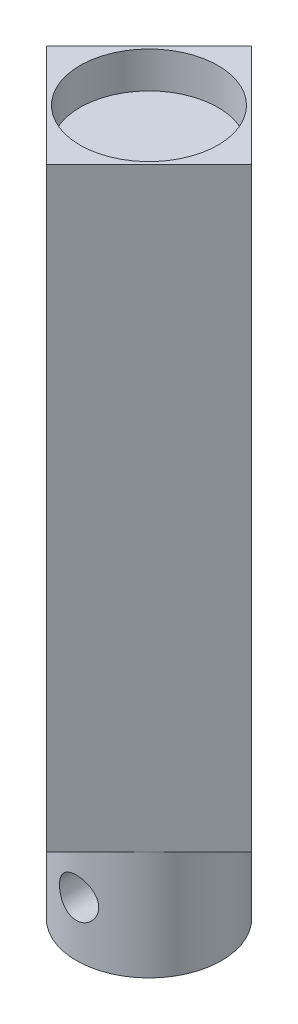
ISO-10303-21;
HEADER;
FILE_DESCRIPTION(('STEP AP214'),'2;1');
FILE_NAME('part.step','',(''),(''),'','','');
FILE_SCHEMA(('AUTOMOTIVE_DESIGN { 1 0 10303 214 1 1 1 1 }'));
ENDSEC;
DATA;
#1=APPLICATION_CONTEXT('core data for automotive mechanical design processes');
#2=APPLICATION_PROTOCOL_DEFINITION('international standard','automotive_design',2000,#1);
#3=PRODUCT_CONTEXT('',#1,'mechanical');
#4=PRODUCT('Part','Part','',(#3));
#5=PRODUCT_RELATED_PRODUCT_CATEGORY('part','',(#4));
#6=PRODUCT_DEFINITION_FORMATION('','',#4);
#7=PRODUCT_DEFINITION_CONTEXT('part definition',#1,'design');
#8=PRODUCT_DEFINITION('design','',#6,#7);
#9=PRODUCT_DEFINITION_SHAPE('','',#8);
#10=(LENGTH_UNIT() NAMED_UNIT(*) SI_UNIT(.MILLI.,.METRE.));
#11=(NAMED_UNIT(*) PLANE_ANGLE_UNIT() SI_UNIT($,.RADIAN.));
#12=(NAMED_UNIT(*) SI_UNIT($,.STERADIAN.) SOLID_ANGLE_UNIT());
#13=UNCERTAINTY_MEASURE_WITH_UNIT(LENGTH_MEASURE(1.E-05),#10,'distance_accuracy_value','');
#14=(GEOMETRIC_REPRESENTATION_CONTEXT(3) GLOBAL_UNCERTAINTY_ASSIGNED_CONTEXT((#13)) GLOBAL_UNIT_ASSIGNED_CONTEXT((#10,
#11,#12)) REPRESENTATION_CONTEXT('',''));
#15=CARTESIAN_POINT('',(0.,0.,0.));
#16=DIRECTION('',(0.,0.,1.));
#17=DIRECTION('',(1.,0.,0.));
#18=AXIS2_PLACEMENT_3D('',#15,#16,#17);
#19=CARTESIAN_POINT('',(0.,0.,0.));
#20=DIRECTION('',(0.,-1.,0.));
#21=DIRECTION('',(0.,0.,-1.));
#22=AXIS2_PLACEMENT_3D('',#19,#20,#21);
#23=PLANE('',#22);
#24=CARTESIAN_POINT('',(0.,0.,0.));
#25=DIRECTION('',(0.,-1.,0.));
#26=DIRECTION('',(0.,0.,-1.));
#27=AXIS2_PLACEMENT_3D('',#24,#25,#26);
#28=CIRCLE('',#27,10.);
#29=CARTESIAN_POINT('',(7.07106781186549,0.,-7.07106781186546));
#30=VERTEX_POINT('',#29);
#31=CARTESIAN_POINT('',(7.07106781186549,0.,7.07106781186546));
#32=VERTEX_POINT('',#31);
#33=EDGE_CURVE('E53',#30,#32,#28,.T.);
#34=ORIENTED_EDGE('',*,*,#33,.F.);
#35=DIRECTION('',(-0.707106781186546,0.,-0.707106781186549));
#36=VECTOR('',#35,1.);
#37=CARTESIAN_POINT('',(14.1421356237309,0.,0.));
#38=LINE('',#37,#36);
#39=CARTESIAN_POINT('',(14.1421356237309,0.,0.));
#40=VERTEX_POINT('',#39);
#41=EDGE_CURVE('E101',#40,#30,#38,.T.);
#42=ORIENTED_EDGE('',*,*,#41,.F.);
#43=DIRECTION('',(0.707106781186546,0.,-0.707106781186549));
#44=VECTOR('',#43,1.);
#45=CARTESIAN_POINT('',(14.1421356237309,0.,0.));
#46=LINE('',#45,#44);
#47=EDGE_CURVE('E117',#32,#40,#46,.T.);
#48=ORIENTED_EDGE('',*,*,#47,.F.);
#49=EDGE_LOOP('',(#34,#42,#48));
#50=FACE_BOUND('',#49,.T.);
#51=ADVANCED_FACE('F43',(#50),#23,.T.);
#52=CARTESIAN_POINT('',(-7.07106781186549,0.,7.07106781186546));
#53=VERTEX_POINT('',#52);
#54=EDGE_CURVE('E11',#32,#53,#28,.T.);
#55=ORIENTED_EDGE('',*,*,#54,.F.);
#56=CARTESIAN_POINT('',(0.,0.,14.142135623731));
#57=VERTEX_POINT('',#56);
#58=EDGE_CURVE('E116',#57,#32,#46,.T.);
#59=ORIENTED_EDGE('',*,*,#58,.F.);
#60=DIRECTION('',(0.707106781186546,0.,0.707106781186549));
#61=VECTOR('',#60,1.);
#62=CARTESIAN_POINT('',(-14.1421356237309,0.,0.));
#63=LINE('',#62,#61);
#64=EDGE_CURVE('E135',#53,#57,#63,.T.);
#65=ORIENTED_EDGE('',*,*,#64,.F.);
#66=EDGE_LOOP('',(#55,#59,#65));
#67=FACE_BOUND('',#66,.T.);
#68=ADVANCED_FACE('F163',(#67),#23,.T.);
#69=CARTESIAN_POINT('',(-7.07106781186549,0.,-7.07106781186546));
#70=VERTEX_POINT('',#69);
#71=EDGE_CURVE('E55',#53,#70,#28,.T.);
#72=ORIENTED_EDGE('',*,*,#71,.F.);
#73=CARTESIAN_POINT('',(-14.1421356237309,0.,0.));
#74=VERTEX_POINT('',#73);
#75=EDGE_CURVE('E148',#74,#53,#63,.T.);
#76=ORIENTED_EDGE('',*,*,#75,.F.);
#77=DIRECTION('',(-0.707106781186546,0.,0.707106781186549));
#78=VECTOR('',#77,1.);
#79=CARTESIAN_POINT('',(-14.1421356237309,0.,0.));
#80=LINE('',#79,#78);
#81=EDGE_CURVE('E112',#70,#74,#80,.T.);
#82=ORIENTED_EDGE('',*,*,#81,.F.);
#83=EDGE_LOOP('',(#72,#76,#82));
#84=FACE_BOUND('',#83,.T.);
#85=ADVANCED_FACE('F169',(#84),#23,.T.);
#86=CARTESIAN_POINT('',(-14.1421356237309,82.,0.));
#87=DIRECTION('',(0.707106781186549,0.,-0.707106781186546));
#88=DIRECTION('',(-0.707106781186546,0.,-0.707106781186549));
#89=AXIS2_PLACEMENT_3D('',#86,#87,#88);
#90=PLANE('',#89);
#91=ORIENTED_EDGE('',*,*,#75,.T.);
#92=ORIENTED_EDGE('',*,*,#64,.T.);
#93=DIRECTION('',(0.,-1.,0.));
#94=VECTOR('',#93,1.);
#95=CARTESIAN_POINT('',(0.,82.,14.142135623731));
#96=LINE('',#95,#94);
#97=CARTESIAN_POINT('',(0.,82.,14.142135623731));
#98=VERTEX_POINT('',#97);
#99=EDGE_CURVE('E50',#98,#57,#96,.T.);
#100=ORIENTED_EDGE('',*,*,#99,.F.);
#101=DIRECTION('',(0.707106781186546,0.,0.707106781186549));
#102=VECTOR('',#101,1.);
#103=CARTESIAN_POINT('',(-14.1421356237309,82.,0.));
#104=LINE('',#103,#102);
#105=CARTESIAN_POINT('',(-14.1421356237309,82.,0.));
#106=VERTEX_POINT('',#105);
#107=EDGE_CURVE('E139',#106,#98,#104,.T.);
#108=ORIENTED_EDGE('',*,*,#107,.F.);
#109=DIRECTION('',(0.,-1.,0.));
#110=VECTOR('',#109,1.);
#111=CARTESIAN_POINT('',(-14.1421356237309,82.,0.));
#112=LINE('',#111,#110);
#113=EDGE_CURVE('E144',#106,#74,#112,.T.);
#114=ORIENTED_EDGE('',*,*,#113,.T.);
#115=EDGE_LOOP('',(#91,#92,#100,#108,#114));
#116=FACE_BOUND('',#115,.T.);
#117=ADVANCED_FACE('F44',(#116),#90,.F.);
#118=CARTESIAN_POINT('',(14.1421356237309,82.,0.));
#119=DIRECTION('',(-0.707106781186549,0.,-0.707106781186546));
#120=DIRECTION('',(-0.707106781186546,0.,0.707106781186549));
#121=AXIS2_PLACEMENT_3D('',#118,#119,#120);
#122=PLANE('',#121);
#123=ORIENTED_EDGE('',*,*,#58,.T.);
#124=ORIENTED_EDGE('',*,*,#47,.T.);
#125=DIRECTION('',(0.,-1.,0.));
#126=VECTOR('',#125,1.);
#127=CARTESIAN_POINT('',(14.1421356237309,82.,0.));
#128=LINE('',#127,#126);
#129=CARTESIAN_POINT('',(14.1421356237309,82.,0.));
#130=VERTEX_POINT('',#129);
#131=EDGE_CURVE('E107',#130,#40,#128,.T.);
#132=ORIENTED_EDGE('',*,*,#131,.F.);
#133=DIRECTION('',(0.707106781186546,0.,-0.707106781186549));
#134=VECTOR('',#133,1.);
#135=CARTESIAN_POINT('',(14.1421356237309,82.,0.));
#136=LINE('',#135,#134);
#137=EDGE_CURVE('E138',#98,#130,#136,.T.);
#138=ORIENTED_EDGE('',*,*,#137,.F.);
#139=ORIENTED_EDGE('',*,*,#99,.T.);
#140=EDGE_LOOP('',(#123,#124,#132,#138,#139));
#141=FACE_BOUND('',#140,.T.);
#142=ADVANCED_FACE('F162',(#141),#122,.F.);
#143=CARTESIAN_POINT('',(14.1421356237309,82.,0.));
#144=DIRECTION('',(-0.707106781186549,0.,0.707106781186546));
#145=DIRECTION('',(0.707106781186546,0.,0.707106781186549));
#146=AXIS2_PLACEMENT_3D('',#143,#144,#145);
#147=PLANE('',#146);
#148=ORIENTED_EDGE('',*,*,#41,.T.);
#149=CARTESIAN_POINT('',(0.,0.,-14.142135623731));
#150=VERTEX_POINT('',#149);
#151=EDGE_CURVE('E102',#30,#150,#38,.T.);
#152=ORIENTED_EDGE('',*,*,#151,.T.);
#153=DIRECTION('',(0.,-1.,0.));
#154=VECTOR('',#153,1.);
#155=CARTESIAN_POINT('',(0.,82.,-14.142135623731));
#156=LINE('',#155,#154);
#157=CARTESIAN_POINT('',(0.,82.,-14.142135623731));
#158=VERTEX_POINT('',#157);
#159=EDGE_CURVE('E153',#158,#150,#156,.T.);
#160=ORIENTED_EDGE('',*,*,#159,.F.);
#161=DIRECTION('',(-0.707106781186546,0.,-0.707106781186549));
#162=VECTOR('',#161,1.);
#163=CARTESIAN_POINT('',(14.1421356237309,82.,0.));
#164=LINE('',#163,#162);
#165=EDGE_CURVE('E143',#130,#158,#164,.T.);
#166=ORIENTED_EDGE('',*,*,#165,.F.);
#167=ORIENTED_EDGE('',*,*,#131,.T.);
#168=EDGE_LOOP('',(#148,#152,#160,#166,#167));
#169=FACE_BOUND('',#168,.T.);
#170=ADVANCED_FACE('F105',(#169),#147,.F.);
#171=CARTESIAN_POINT('',(-14.1421356237309,82.,0.));
#172=DIRECTION('',(0.707106781186549,0.,0.707106781186546));
#173=DIRECTION('',(0.707106781186546,0.,-0.707106781186549));
#174=AXIS2_PLACEMENT_3D('',#171,#172,#173);
#175=PLANE('',#174);
#176=EDGE_CURVE('E113',#150,#70,#80,.T.);
#177=ORIENTED_EDGE('',*,*,#176,.T.);
#178=ORIENTED_EDGE('',*,*,#81,.T.);
#179=ORIENTED_EDGE('',*,*,#113,.F.);
#180=DIRECTION('',(-0.707106781186546,0.,0.707106781186549));
#181=VECTOR('',#180,1.);
#182=CARTESIAN_POINT('',(-14.1421356237309,82.,0.));
#183=LINE('',#182,#181);
#184=EDGE_CURVE('E141',#158,#106,#183,.T.);
#185=ORIENTED_EDGE('',*,*,#184,.F.);
#186=ORIENTED_EDGE('',*,*,#159,.T.);
#187=EDGE_LOOP('',(#177,#178,#179,#185,#186));
#188=FACE_BOUND('',#187,.T.);
#189=ADVANCED_FACE('F156',(#188),#175,.F.);
#190=CARTESIAN_POINT('',(0.,82.,0.));
#191=DIRECTION('',(0.,-1.,0.));
#192=DIRECTION('',(0.,0.,-1.));
#193=AXIS2_PLACEMENT_3D('',#190,#191,#192);
#194=PLANE('',#193);
#195=CARTESIAN_POINT('',(0.,82.,0.));
#196=DIRECTION('',(0.,1.,0.));
#197=DIRECTION('',(0.,0.,1.));
#198=AXIS2_PLACEMENT_3D('',#195,#196,#197);
#199=CIRCLE('',#198,9.5);
#200=CARTESIAN_POINT('',(0.,82.,9.5));
#201=VERTEX_POINT('',#200);
#202=EDGE_CURVE('E132',#201,#201,#199,.T.);
#203=ORIENTED_EDGE('',*,*,#202,.F.);
#204=EDGE_LOOP('',(#203));
#205=FACE_BOUND('',#204,.T.);
#206=ORIENTED_EDGE('',*,*,#107,.T.);
#207=ORIENTED_EDGE('',*,*,#137,.T.);
#208=ORIENTED_EDGE('',*,*,#165,.T.);
#209=ORIENTED_EDGE('',*,*,#184,.T.);
#210=EDGE_LOOP('',(#206,#207,#208,#209));
#211=FACE_BOUND('',#210,.T.);
#212=ADVANCED_FACE('F157',(#205,#211),#194,.F.);
#213=EDGE_CURVE('E66',#70,#30,#28,.T.);
#214=ORIENTED_EDGE('',*,*,#213,.F.);
#215=ORIENTED_EDGE('',*,*,#176,.F.);
#216=ORIENTED_EDGE('',*,*,#151,.F.);
#217=EDGE_LOOP('',(#214,#215,#216));
#218=FACE_BOUND('',#217,.T.);
#219=ADVANCED_FACE('F114',(#218),#23,.T.);
#220=CARTESIAN_POINT('',(0.,77.,0.));
#221=DIRECTION('',(0.,1.,0.));
#222=DIRECTION('',(0.,0.,1.));
#223=AXIS2_PLACEMENT_3D('',#220,#221,#222);
#224=CYLINDRICAL_SURFACE('',#223,9.5);
#225=CARTESIAN_POINT('',(0.,77.,0.));
#226=DIRECTION('',(0.,1.,0.));
#227=DIRECTION('',(0.,0.,1.));
#228=AXIS2_PLACEMENT_3D('',#225,#226,#227);
#229=CIRCLE('',#228,9.5);
#230=CARTESIAN_POINT('',(0.,77.,9.5));
#231=VERTEX_POINT('',#230);
#232=EDGE_CURVE('E129',#231,#231,#229,.T.);
#233=ORIENTED_EDGE('',*,*,#232,.F.);
#234=EDGE_LOOP('',(#233));
#235=FACE_BOUND('',#234,.T.);
#236=ORIENTED_EDGE('',*,*,#202,.T.);
#237=EDGE_LOOP('',(#236));
#238=FACE_BOUND('',#237,.T.);
#239=ADVANCED_FACE('F180',(#235,#238),#224,.F.);
#240=CARTESIAN_POINT('',(0.,77.,0.));
#241=DIRECTION('',(0.,1.,0.));
#242=DIRECTION('',(0.,0.,1.));
#243=AXIS2_PLACEMENT_3D('',#240,#241,#242);
#244=PLANE('',#243);
#245=ORIENTED_EDGE('',*,*,#232,.T.);
#246=EDGE_LOOP('',(#245));
#247=FACE_BOUND('',#246,.T.);
#248=ADVANCED_FACE('F190',(#247),#244,.T.);
#249=CARTESIAN_POINT('',(0.,-15.,0.));
#250=DIRECTION('',(0.,1.,0.));
#251=DIRECTION('',(0.,0.,1.));
#252=AXIS2_PLACEMENT_3D('',#249,#250,#251);
#253=CYLINDRICAL_SURFACE('',#252,10.);
#254=CARTESIAN_POINT('',(0.,-10.2051,10.));
#255=CARTESIAN_POINT('',(-0.149045037083741,-10.2050966299615,9.99999783430908));
#256=CARTESIAN_POINT('',(-0.298125866052346,-10.1927406665123,9.99663514499211));
#257=CARTESIAN_POINT('',(-0.591987739591023,-10.1437339962595,9.98354748189365));
#258=CARTESIAN_POINT('',(-0.736766770221911,-10.1070720918998,9.97381957573374));
#259=CARTESIAN_POINT('',(-1.01774119287178,-10.0107366072679,9.94907433569422));
#260=CARTESIAN_POINT('',(-1.1539475599675,-9.95109317596493,9.93406393403307));
#261=CARTESIAN_POINT('',(-1.41442441616562,-9.81060079085221,9.90033712566658));
#262=CARTESIAN_POINT('',(-1.53869401762973,-9.72975026171161,9.88162044367224));
#263=CARTESIAN_POINT('',(-1.77472745738721,-9.54710747633259,9.84200106131268));
#264=CARTESIAN_POINT('',(-1.88616673669218,-9.44490406877735,9.82106014969195));
#265=CARTESIAN_POINT('',(-2.09055098982339,-9.22333531336752,9.77959586314569));
#266=CARTESIAN_POINT('',(-2.18349350879342,-9.10396769112615,9.75907254396633));
#267=CARTESIAN_POINT('',(-2.349842023944,-8.84885128463224,9.72037488270877));
#268=CARTESIAN_POINT('',(-2.42287215807647,-8.71284944615689,9.7022486749669));
#269=CARTESIAN_POINT('',(-2.54490097280709,-8.42992776216281,9.67096040737312));
#270=CARTESIAN_POINT('',(-2.59390422793279,-8.28301000108794,9.65779740267694));
#271=CARTESIAN_POINT('',(-2.66535632074227,-7.9860272008663,9.63832082351118));
#272=CARTESIAN_POINT('',(-2.68839473242032,-7.83611420922625,9.63185545614462));
#273=CARTESIAN_POINT('',(-2.70910160304402,-7.53442236407939,9.62605287536555));
#274=CARTESIAN_POINT('',(-2.70677495179707,-7.38264387583299,9.62671428807159));
#275=CARTESIAN_POINT('',(-2.67728525199069,-7.08615172917667,9.63495482234529));
#276=CARTESIAN_POINT('',(-2.65083828361374,-6.94136041868448,9.64233448226496));
#277=CARTESIAN_POINT('',(-2.57500667724389,-6.65835086609988,9.66286027172692));
#278=CARTESIAN_POINT('',(-2.52562015863842,-6.52013316394431,9.67600687404534));
#279=CARTESIAN_POINT('',(-2.4047341294501,-6.25234049981045,9.70675883733144));
#280=CARTESIAN_POINT('',(-2.33298567026911,-6.12288387447025,9.72441396928952));
#281=CARTESIAN_POINT('',(-2.16958602322398,-5.87759746603615,9.76216726353275));
#282=CARTESIAN_POINT('',(-2.07793081527352,-5.76177044267951,9.78226591891599));
#283=CARTESIAN_POINT('',(-1.8736695430037,-5.54294299162871,9.82346959072877));
#284=CARTESIAN_POINT('',(-1.76046289348824,-5.44050445697942,9.84458572771544));
#285=CARTESIAN_POINT('',(-1.51821873144213,-5.25594923301467,9.8848401839404));
#286=CARTESIAN_POINT('',(-1.38918055895671,-5.17383339130425,9.90397842066638));
#287=CARTESIAN_POINT('',(-1.11804965365092,-5.03199711605937,9.93824415703912));
#288=CARTESIAN_POINT('',(-0.975899892120033,-4.97238086989606,9.95335290524466));
#289=CARTESIAN_POINT('',(-0.683092985514605,-4.87805539347203,9.97772189394846));
#290=CARTESIAN_POINT('',(-0.532437763476409,-4.84334055727798,9.98698345074018));
#291=CARTESIAN_POINT('',(-0.231689723497275,-4.80069137629116,9.99841445628651));
#292=CARTESIAN_POINT('',(-0.081712720487699,-4.79199337323195,10.0007860798073));
#293=CARTESIAN_POINT('',(0.21755793620496,-4.79951237065665,9.99875256684006));
#294=CARTESIAN_POINT('',(0.366851661027029,-4.81572671536809,9.99434815270918));
#295=CARTESIAN_POINT('',(0.657775057501917,-4.87198461746751,9.97938825604903));
#296=CARTESIAN_POINT('',(0.799493738342592,-4.9116000038541,9.9689433669295));
#297=CARTESIAN_POINT('',(1.07425843612871,-5.01303628206868,9.943089497538));
#298=CARTESIAN_POINT('',(1.20730349771939,-5.07485961512251,9.92767997154367));
#299=CARTESIAN_POINT('',(1.46389444444125,-5.2203583280213,9.89313506683897));
#300=CARTESIAN_POINT('',(1.58719698709217,-5.30444620371536,9.87393130532195));
#301=CARTESIAN_POINT('',(1.8182087533198,-5.49157047249854,9.83401662833237));
#302=CARTESIAN_POINT('',(1.92591479633399,-5.59461072080785,9.81330540673688));
#303=CARTESIAN_POINT('',(2.12591059516576,-5.82028211316183,9.77196254366284));
#304=CARTESIAN_POINT('',(2.2176609227028,-5.94339585081846,9.75135073319754));
#305=CARTESIAN_POINT('',(2.37921420847329,-6.2037103431043,9.71320009738658));
#306=CARTESIAN_POINT('',(2.44901805964973,-6.3409105242927,9.69566114702738));
#307=CARTESIAN_POINT('',(2.56417282388669,-6.62483726084514,9.66584491556549));
#308=CARTESIAN_POINT('',(2.60966358932046,-6.77150377213331,9.65353762687842));
#309=CARTESIAN_POINT('',(2.67521992497626,-7.07079579710599,9.63557863666349));
#310=CARTESIAN_POINT('',(2.69529222402635,-7.22341972269891,9.62992517374935));
#311=CARTESIAN_POINT('',(2.70904663644172,-7.52476304354507,9.62606407537705));
#312=CARTESIAN_POINT('',(2.70359700230998,-7.67344025414247,9.62761145666402));
#313=CARTESIAN_POINT('',(2.66848271435519,-7.9676709357749,9.63740241610983));
#314=CARTESIAN_POINT('',(2.63881871836108,-8.11322449155969,9.64564581235874));
#315=CARTESIAN_POINT('',(2.55662781281297,-8.39594770401969,9.66775201958407));
#316=CARTESIAN_POINT('',(2.50428992476036,-8.53317620627412,9.68156830773152));
#317=CARTESIAN_POINT('',(2.37838344924478,-8.79700935833853,9.71326349704956));
#318=CARTESIAN_POINT('',(2.30481144390359,-8.92361229360188,9.73114305215167));
#319=CARTESIAN_POINT('',(2.13591514407799,-9.16673247380289,9.76962495218788));
#320=CARTESIAN_POINT('',(2.04000077553741,-9.2828294021125,9.79029324275764));
#321=CARTESIAN_POINT('',(1.83025798760164,-9.49756226394294,9.83166122402304));
#322=CARTESIAN_POINT('',(1.71642519052025,-9.59619391794283,9.85236092116455));
#323=CARTESIAN_POINT('',(1.47102699787676,-9.77535312979699,9.89200929131388));
#324=CARTESIAN_POINT('',(1.33912395253035,-9.85543001199162,9.91090887152721));
#325=CARTESIAN_POINT('',(1.06322026132516,-9.99214735734186,9.94428547063828));
#326=CARTESIAN_POINT('',(0.919227222943829,-10.0488024273736,9.95876524444349));
#327=CARTESIAN_POINT('',(0.64653431690388,-10.1299266460811,9.97986362493178));
#328=CARTESIAN_POINT('',(0.518977619094993,-10.1580500424681,9.98735895853281));
#329=CARTESIAN_POINT('',(0.2609562214406,-10.1956372144808,9.99742783557166));
#330=CARTESIAN_POINT('',(0.13049182857407,-10.2051029505342,10.0000018961045));
#331=CARTESIAN_POINT('',(0.,-10.2051,10.));
#332=B_SPLINE_CURVE_WITH_KNOTS('',3,(#254,#255,#256,#257,#258,#259,#260,#261,#262,#263,#264,
#265,#266,#267,#268,#269,#270,#271,#272,#273,#274,#275,#276,#277,#278,#279,#280,#281,#282,#283,
#284,#285,#286,#287,#288,#289,#290,#291,#292,#293,#294,#295,#296,#297,#298,#299,#300,#301,#302,
#303,#304,#305,#306,#307,#308,#309,#310,#311,#312,#313,#314,#315,#316,#317,#318,#319,#320,#321,
#322,#323,#324,#325,#326,#327,#328,#329,#330,#331),.UNSPECIFIED.,.T.,.F.,(4,2,2,2,2,2,2,2,2,2,2,
2,2,2,2,2,2,2,2,2,2,2,2,2,2,2,2,2,2,2,2,2,2,2,2,2,2,2,4),(0.,0.446656480142376,
0.893518874535914,1.33979702482449,1.7861083354693,2.241971337888,2.69789480132285,
3.16190703418501,3.62583088845321,4.07899386792752,4.53206948942802,4.97211717933805,
5.41220095126816,5.85737045706276,6.30262994674247,6.7628535113881,7.2230962674914,
7.68544482593925,8.1476892654098,8.59622562760989,9.044714177059,9.48524032833899,
9.92581491962561,10.3752051916181,10.8246869781857,11.2872405538501,11.7497753070195,
12.2096200507985,12.6693430380783,13.1135421599348,13.5577292146836,13.9982824772784,
14.438906691632,14.8928442628531,15.3468929090699,15.8110245673828,16.2748663344566,
16.6659638655521,17.0570203004301),.UNSPECIFIED.);
#333=CARTESIAN_POINT('',(0.,-10.2051,10.));
#334=VERTEX_POINT('',#333);
#335=EDGE_CURVE('E270',#334,#334,#332,.T.);
#336=ORIENTED_EDGE('',*,*,#335,.T.);
#337=EDGE_LOOP('',(#336));
#338=FACE_BOUND('',#337,.T.);
#339=CARTESIAN_POINT('',(0.,-15.,0.));
#340=DIRECTION('',(0.,-1.,0.));
#341=DIRECTION('',(0.,0.,-1.));
#342=AXIS2_PLACEMENT_3D('',#339,#340,#341);
#343=CIRCLE('',#342,10.);
#344=CARTESIAN_POINT('',(0.,-15.,-10.));
#345=VERTEX_POINT('',#344);
#346=EDGE_CURVE('E124',#345,#345,#343,.T.);
#347=ORIENTED_EDGE('',*,*,#346,.F.);
#348=EDGE_LOOP('',(#347));
#349=FACE_BOUND('',#348,.T.);
#350=ORIENTED_EDGE('',*,*,#33,.T.);
#351=ORIENTED_EDGE('',*,*,#54,.T.);
#352=ORIENTED_EDGE('',*,*,#71,.T.);
#353=ORIENTED_EDGE('',*,*,#213,.T.);
#354=EDGE_LOOP('',(#350,#351,#352,#353));
#355=FACE_BOUND('',#354,.T.);
#356=ADVANCED_FACE('F123',(#338,#349,#355),#253,.T.);
#357=CARTESIAN_POINT('',(0.,-15.,0.));
#358=DIRECTION('',(0.,-1.,0.));
#359=DIRECTION('',(0.,0.,-1.));
#360=AXIS2_PLACEMENT_3D('',#357,#358,#359);
#361=PLANE('',#360);
#362=CARTESIAN_POINT('',(0.,-15.,0.));
#363=DIRECTION('',(0.,-1.,0.));
#364=DIRECTION('',(0.,0.,-1.));
#365=AXIS2_PLACEMENT_3D('',#362,#363,#364);
#366=CIRCLE('',#365,6.);
#367=CARTESIAN_POINT('',(0.,-15.,-6.));
#368=VERTEX_POINT('',#367);
#369=EDGE_CURVE('E121',#368,#368,#366,.T.);
#370=ORIENTED_EDGE('',*,*,#369,.F.);
#371=EDGE_LOOP('',(#370));
#372=FACE_BOUND('',#371,.T.);
#373=ORIENTED_EDGE('',*,*,#346,.T.);
#374=EDGE_LOOP('',(#373));
#375=FACE_BOUND('',#374,.T.);
#376=ADVANCED_FACE('F210',(#372,#375),#361,.T.);
#377=CARTESIAN_POINT('',(0.,-15.,0.));
#378=DIRECTION('',(0.,1.,0.));
#379=DIRECTION('',(0.,0.,1.));
#380=AXIS2_PLACEMENT_3D('',#377,#378,#379);
#381=CYLINDRICAL_SURFACE('',#380,6.);
#382=CARTESIAN_POINT('',(0.,-10.2051,6.));
#383=CARTESIAN_POINT('',(-0.143830249000788,-10.2050918852,5.99999338999734));
#384=CARTESIAN_POINT('',(-0.287884014569675,-10.1935605526752,5.99477026081526));
#385=CARTESIAN_POINT('',(-0.571832719631682,-10.1478953843536,5.97439376881437));
#386=CARTESIAN_POINT('',(-0.711717073008222,-10.1137084155209,5.95921706327962));
#387=CARTESIAN_POINT('',(-0.982774255664464,-10.0242837493316,5.92054300913512));
#388=CARTESIAN_POINT('',(-1.11397653057179,-9.96912199313326,5.8970756989066));
#389=CARTESIAN_POINT('',(-1.36511532100493,-9.83965827045813,5.84405301949512));
#390=CARTESIAN_POINT('',(-1.48505420132938,-9.76536033402087,5.8144989324369));
#391=CARTESIAN_POINT('',(-1.71728016431582,-9.5953015061785,5.75032238409619));
#392=CARTESIAN_POINT('',(-1.82884653125863,-9.49862646224672,5.71551642976307));
#393=CARTESIAN_POINT('',(-2.034821320312,-9.28850104995766,5.64547255717065));
#394=CARTESIAN_POINT('',(-2.12921921691739,-9.17504046763008,5.61023438796729));
#395=CARTESIAN_POINT('',(-2.30379400028296,-8.92636797767458,5.54092810093915));
#396=CARTESIAN_POINT('',(-2.38278202655822,-8.79026080042798,5.50705614966236));
#397=CARTESIAN_POINT('',(-2.51642362568589,-8.50496207765698,5.44729385057242));
#398=CARTESIAN_POINT('',(-2.57109179061533,-8.35577844259578,5.42139871949125));
#399=CARTESIAN_POINT('',(-2.65144214864756,-8.05683511703704,5.38254234609388));
#400=CARTESIAN_POINT('',(-2.67852042195821,-7.90753453754741,5.36896246634564));
#401=CARTESIAN_POINT('',(-2.70725789454398,-7.60593991695485,5.35453471904145));
#402=CARTESIAN_POINT('',(-2.70893484105389,-7.4536480402879,5.35367796218446));
#403=CARTESIAN_POINT('',(-2.6878610501444,-7.16549936571074,5.36427908853507));
#404=CARTESIAN_POINT('',(-2.66735955202031,-7.02942733470839,5.37460316844463));
#405=CARTESIAN_POINT('',(-2.60633220887016,-6.76291408182894,5.40445872048247));
#406=CARTESIAN_POINT('',(-2.56580168937545,-6.63247418213668,5.42399234192863));
#407=CARTESIAN_POINT('',(-2.46506452262258,-6.37738532212081,5.47051938288511));
#408=CARTESIAN_POINT('',(-2.404432896112,-6.25293451602923,5.4976717854472));
#409=CARTESIAN_POINT('',(-2.26552187878021,-6.01543841293758,5.55635564318898));
#410=CARTESIAN_POINT('',(-2.18723496675836,-5.90239800659589,5.58788896244669));
#411=CARTESIAN_POINT('',(-2.00601869088672,-5.67896538794809,5.65562943998153));
#412=CARTESIAN_POINT('',(-1.90140299775264,-5.56998242441241,5.6919877347948));
#413=CARTESIAN_POINT('',(-1.67508998063358,-5.37058879571416,5.76264879265146));
#414=CARTESIAN_POINT('',(-1.55338721456383,-5.28018407024821,5.79695089582949));
#415=CARTESIAN_POINT('',(-1.29144480165142,-5.11794499521687,5.86096256316377));
#416=CARTESIAN_POINT('',(-1.1507452272809,-5.04677814937102,5.89049542002625));
#417=CARTESIAN_POINT('',(-0.857697251110994,-4.92963519342281,5.94023401201306));
#418=CARTESIAN_POINT('',(-0.705356481156393,-4.88364273800723,5.96044579780812));
#419=CARTESIAN_POINT('',(-0.405042420485967,-4.82132122892515,5.98807450330902));
#420=CARTESIAN_POINT('',(-0.257535245787298,-4.80310691495507,5.99630269313837));
#421=CARTESIAN_POINT('',(0.0386492460318007,-4.79112274465748,6.00170084658227));
#422=CARTESIAN_POINT('',(0.187326131595395,-4.79734425948518,5.99887471373007));
#423=CARTESIAN_POINT('',(0.472172217005337,-4.83279517755675,5.98299222685402));
#424=CARTESIAN_POINT('',(0.608555724216769,-4.86061764516769,5.97056166881312));
#425=CARTESIAN_POINT('',(0.87452095912351,-4.93642669546325,5.93743915230051));
#426=CARTESIAN_POINT('',(1.00410186661765,-4.98441570340964,5.91674620019445));
#427=CARTESIAN_POINT('',(1.25736918355507,-5.10070571887961,5.86823428740504));
#428=CARTESIAN_POINT('',(1.38074691964035,-5.16959204210287,5.84021371286274));
#429=CARTESIAN_POINT('',(1.61463545552275,-5.32508349864137,5.77992761361742));
#430=CARTESIAN_POINT('',(1.72514059071439,-5.41169638668161,5.74766023330451));
#431=CARTESIAN_POINT('',(1.93978772735996,-5.60851748656145,5.67899197137962));
#432=CARTESIAN_POINT('',(2.04264796218825,-5.72008457027095,5.64246992340334));
#433=CARTESIAN_POINT('',(2.22863389789407,-5.95931076819581,5.5716350928417));
#434=CARTESIAN_POINT('',(2.31175193981723,-6.08697609839419,5.5373231714216));
#435=CARTESIAN_POINT('',(2.45776198652826,-6.35920017248153,5.47411371164458));
#436=CARTESIAN_POINT('',(2.52007386270723,-6.50411103353912,5.44537957440296));
#437=CARTESIAN_POINT('',(2.61880527539143,-6.80408952347694,5.39860129485975));
#438=CARTESIAN_POINT('',(2.65525110372609,-6.95914666340304,5.38054630074521));
#439=CARTESIAN_POINT('',(2.69840660396585,-7.26059660368905,5.35902325322731));
#440=CARTESIAN_POINT('',(2.70741352734677,-7.4065804192937,5.35442961207842));
#441=CARTESIAN_POINT('',(2.701776495782,-7.69795349988541,5.35727722162229));
#442=CARTESIAN_POINT('',(2.68713799440377,-7.84334289421638,5.36471569723498));
#443=CARTESIAN_POINT('',(2.6366544010182,-8.11976670055273,5.3896900477912));
#444=CARTESIAN_POINT('',(2.60221863334447,-8.25112574832216,5.40655298249864));
#445=CARTESIAN_POINT('',(2.51463242914749,-8.50617310255179,5.44783945559982));
#446=CARTESIAN_POINT('',(2.46147654112442,-8.62985916220203,5.47226519611311));
#447=CARTESIAN_POINT('',(2.33402464638194,-8.87483803911143,5.52787958150228));
#448=CARTESIAN_POINT('',(2.2585818711682,-8.99545629196171,5.55940392126891));
#449=CARTESIAN_POINT('',(2.0901642081627,-9.22303273148147,5.62488897257464));
#450=CARTESIAN_POINT('',(1.99718173387022,-9.32998497344562,5.65885073442674));
#451=CARTESIAN_POINT('',(1.78630854614247,-9.5372657135336,5.72909419971941));
#452=CARTESIAN_POINT('',(1.66692050898236,-9.63610361436444,5.76530545994353));
#453=CARTESIAN_POINT('',(1.4120470514997,-9.81251671315132,5.83296849739319));
#454=CARTESIAN_POINT('',(1.27655425930247,-9.89008211957966,5.86441807989029));
#455=CARTESIAN_POINT('',(0.99406726289993,-10.0205742202095,5.91880226937506));
#456=CARTESIAN_POINT('',(0.847198238139981,-10.073734030518,5.94181699729363));
#457=CARTESIAN_POINT('',(0.621148623044834,-10.1339779978237,5.968247056316));
#458=CARTESIAN_POINT('',(0.544904809006051,-10.1508043005724,5.97570564386212));
#459=CARTESIAN_POINT('',(0.391042808246186,-10.1778227382942,5.98773876353244));
#460=CARTESIAN_POINT('',(0.313425601226102,-10.1880194208638,5.99231527255425));
#461=CARTESIAN_POINT('',(0.196346620219844,-10.1982511180827,5.99691464700618));
#462=CARTESIAN_POINT('',(0.157131698073632,-10.2008178251188,5.99807023452824));
#463=CARTESIAN_POINT('',(0.0786167520166226,-10.2042433871488,5.99961381983961));
#464=CARTESIAN_POINT('',(0.0393167269215665,-10.2051022182217,6.0000018068777));
#465=CARTESIAN_POINT('',(0.,-10.2051,6.));
#466=B_SPLINE_CURVE_WITH_KNOTS('',3,(#382,#383,#384,#385,#386,#387,#388,#389,#390,#391,#392,
#393,#394,#395,#396,#397,#398,#399,#400,#401,#402,#403,#404,#405,#406,#407,#408,#409,#410,#411,
#412,#413,#414,#415,#416,#417,#418,#419,#420,#421,#422,#423,#424,#425,#426,#427,#428,#429,#430,
#431,#432,#433,#434,#435,#436,#437,#438,#439,#440,#441,#442,#443,#444,#445,#446,#447,#448,#449,
#450,#451,#452,#453,#454,#455,#456,#457,#458,#459,#460,#461,#462,#463,#464,#465),.UNSPECIFIED.,
.T.,.F.,(4,2,2,2,2,2,2,2,2,2,2,2,2,2,2,2,2,2,2,2,2,2,2,2,2,2,2,2,2,2,2,2,2,2,2,2,2,2,2,2,2,4),
(0.,0.431337122573568,0.86368943372029,1.2944910529268,1.72520202029162,2.1782780025413,
2.63163082340678,3.11210966282447,3.59229982165566,4.04676234473427,4.50090733221811,
4.91296807860864,5.32512503915442,5.74661985062268,6.16829456037365,6.63237032617875,
7.09659423280592,7.57530392730755,8.05370243374812,8.49790680192733,8.94195432558487,
9.35928301563545,9.77666190869976,10.2070219588776,10.6375706798331,11.1037215653093,
11.5700529990271,12.0484722599053,12.5264045270579,12.963041117427,13.3995770165569,
13.8083232513679,14.217188616027,14.6525511102927,15.0881023468441,15.5633248793187,
16.0387657864966,16.5095657536734,16.7445873256236,16.9794475136658,17.0973540489947,
17.2152622357439),.UNSPECIFIED.);
#467=CARTESIAN_POINT('',(0.,-10.2051,6.));
#468=VERTEX_POINT('',#467);
#469=EDGE_CURVE('E265',#468,#468,#466,.T.);
#470=ORIENTED_EDGE('',*,*,#469,.F.);
#471=EDGE_LOOP('',(#470));
#472=FACE_BOUND('',#471,.T.);
#473=ORIENTED_EDGE('',*,*,#369,.T.);
#474=EDGE_LOOP('',(#473));
#475=FACE_BOUND('',#474,.T.);
#476=CARTESIAN_POINT('',(0.,0.,0.));
#477=DIRECTION('',(0.,-1.,0.));
#478=DIRECTION('',(0.,0.,-1.));
#479=AXIS2_PLACEMENT_3D('',#476,#477,#478);
#480=CIRCLE('',#479,6.);
#481=CARTESIAN_POINT('',(0.,0.,-6.));
#482=VERTEX_POINT('',#481);
#483=EDGE_CURVE('E272',#482,#482,#480,.T.);
#484=ORIENTED_EDGE('',*,*,#483,.F.);
#485=EDGE_LOOP('',(#484));
#486=FACE_BOUND('',#485,.T.);
#487=ADVANCED_FACE('F218',(#472,#475,#486),#381,.F.);
#488=CARTESIAN_POINT('',(0.,0.,0.));
#489=DIRECTION('',(0.,-1.,0.));
#490=DIRECTION('',(0.,0.,-1.));
#491=AXIS2_PLACEMENT_3D('',#488,#489,#490);
#492=PLANE('',#491);
#493=ORIENTED_EDGE('',*,*,#483,.T.);
#494=EDGE_LOOP('',(#493));
#495=FACE_BOUND('',#494,.T.);
#496=ADVANCED_FACE('F227',(#495),#492,.T.);
#497=CARTESIAN_POINT('',(0.,-7.5,10.));
#498=DIRECTION('',(0.,0.,1.));
#499=DIRECTION('',(1.,0.,0.));
#500=AXIS2_PLACEMENT_3D('',#497,#498,#499);
#501=CYLINDRICAL_SURFACE('',#500,2.70509999999999);
#502=ORIENTED_EDGE('',*,*,#469,.T.);
#503=EDGE_LOOP('',(#502));
#504=FACE_BOUND('',#503,.T.);
#505=ORIENTED_EDGE('',*,*,#335,.F.);
#506=EDGE_LOOP('',(#505));
#507=FACE_BOUND('',#506,.T.);
#508=ADVANCED_FACE('F236',(#504,#507),#501,.F.);
#509=CLOSED_SHELL('',(#51,#68,#85,#117,#142,#170,#189,#212,#219,#239,#248,#356,#376,#487,#496,#508));
#510=MANIFOLD_SOLID_BREP('B2',#509);
#511=ADVANCED_BREP_SHAPE_REPRESENTATION('',(#18,#510),#14);
#512=SHAPE_DEFINITION_REPRESENTATION(#9,#511);
ENDSEC;
END-ISO-10303-21;
